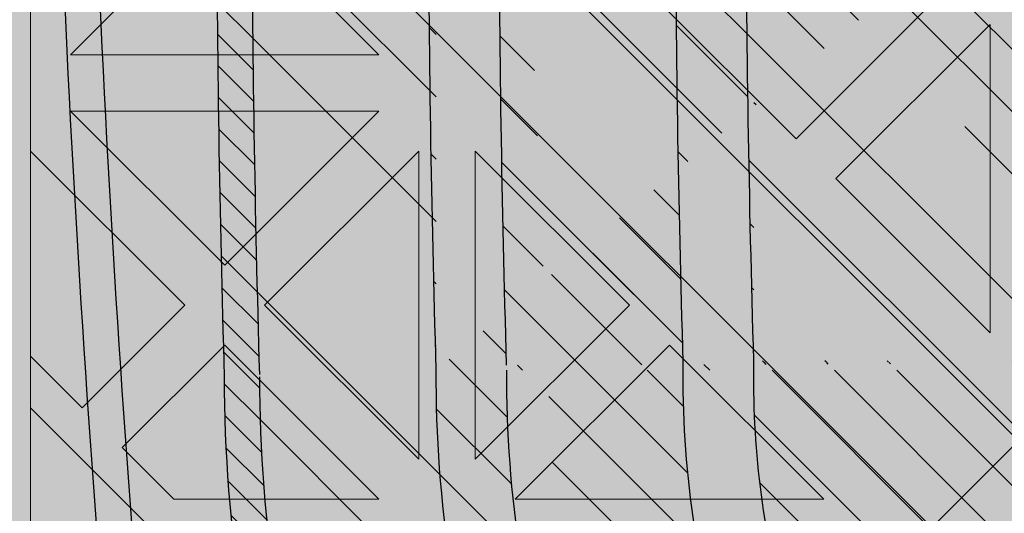
# Model space of a CAD drawing. Units: inches. Extents: x 844 to 2234, y 346 to 1084.
# Tile 28 of 93: x 1252.862 to 1257.311, y 691.183 to 693.415. Entities that reach past the tile are written whole.
import ezdxf

# ---------------------------------------------------------------- set-up
doc = ezdxf.new("R2010")
doc.units = ezdxf.units.IN
doc.header["$MEASUREMENT"] = 0
doc.layers.add('furniture', color=8, linetype='Continuous', lineweight=18)
doc.layers.add('RA-AP-01$0$INT', color=35, linetype='Continuous', lineweight=5)
doc.layers.add('RA-AP-01$0$FURN', color=3, linetype='Continuous')
doc.layers.add('RA-AP-01$0$WOOD', color=64, linetype='Continuous')

# ---------------------------------------------------------------- blocks, each defined once
blk = doc.blocks.new('A$C18D01794')
at = {"layer": 'RA-AP-01$0$INT'}
blk.add_hatch(color=256, dxfattribs=at).paths.add_polyline_path([(4.505206456958071, -6.306712009588038), (5.305206456958072, -6.306712009588038), (5.305206456958072, -7.106712009588038), (5.255206456951893, -7.10671200958804), (5.25520645694868, -6.356712009605972), (4.555206456959269, -6.356712009587461), (4.555206456956052, -7.106712009588038), (4.505206456958073, -7.106712009588038)])
h = blk.add_hatch(color=256, dxfattribs=at)
h.paths.add_polyline_path([(4.585917135068449, -6.356712009588271), (4.555206456959269, -6.35671200958746), (4.555206456959137, -6.387422687716308), (4.874495778835233, -6.706712009592356), (4.90520645695423, -6.676001331474049)])
h.paths.add_polyline_path([(5.255206456948813, -6.387422687716306), (5.255206456948682, -6.356712009605972), (5.224495778822613, -6.356712009605161), (4.905206456953498, -6.676001331474273), (4.935917135072151, -6.706712009592924)])
h.paths.add_polyline_path([(4.935917135072559, -6.706712009592068), (4.905206456953564, -6.737422687710376), (5.255206456951813, -7.087422687708613), (5.255206456951549, -7.026001331471008)])
h.paths.add_polyline_path([(4.555206456956399, -7.026001331471013), (4.555206456956134, -7.087422687708616), (4.905206456953821, -6.737422687710943), (4.874495778835166, -6.70671200959229)])
h = blk.add_hatch(color=256, dxfattribs=at)
h.paths.add_polyline_path([(4.585917135068448, -6.356712009588273), (4.614201406330596, -6.356712009589021), (4.668846067270487, -6.411356670531338), (4.723490728212344, -6.356712009591912), (4.771774999457151, -6.35671200959319), (4.826419660396886, -6.411356670535356), (4.862780050090322, -6.374996280843536), (4.844495778842715, -6.356712009595112), (4.862780050090411, -6.356712009595595), (4.905206456960182, -6.399138416468211), (4.947632863832445, -6.356712009597838), (4.965917135079675, -6.356712009598322), (4.947632863831759, -6.374996280845421), (4.983993253523576, -6.411356670538857), (5.038637914464627, -6.356712009600247), (5.08692218571208, -6.356712009601523), (5.141566846649976, -6.411356670541852), (5.196211507589851, -6.356712009604411), (5.224495778822615, -6.356712009605161), (4.905206456953975, -6.676001331473793)])
h.paths.add_polyline_path([(4.895206456956031, -6.637717060225675), (4.895206456958921, -6.528427738347902), (4.840561796018589, -6.583072399285802)], flags=16)
h.paths.add_polyline_path([(4.915206456955638, -6.637717060226121), (4.969851117895509, -6.583072399288678), (4.915206456957609, -6.528427738348344)], flags=16)
h.paths.add_polyline_path([(4.826419660395175, -6.568930263661755), (4.881064321335613, -6.514285602723745), (4.771774999456703, -6.514285602720857)], flags=16)
h.paths.add_polyline_path([(4.983993253519558, -6.568930263665262), (5.038637914460456, -6.514285602726792), (4.929348592581548, -6.514285602724816)], flags=16)
h.paths.add_polyline_path([(4.881064321336025, -6.494285602723742), (4.826419660397532, -6.439640941782821), (4.771774999457062, -6.494285602720859)], flags=16)
h.paths.add_polyline_path([(4.929348592582019, -6.494285602724817), (5.038637914460982, -6.494285602726792), (4.983993253522945, -6.439640941786327)], flags=16)
h.paths.add_polyline_path([(4.895206456960191, -6.480143467100443), (4.895206456962115, -6.407422687715913), (4.876922185715016, -6.389138416467584), (4.840561796021581, -6.425498806159401)], flags=16)
h.paths.add_polyline_path([(4.915206456958487, -6.480143467100889), (4.969851117899527, -6.425498806162279), (4.933490728206909, -6.389138416468043), (4.9152064569598, -6.40742268771434)], flags=16)
h.paths.add_polyline_path([(4.757632863832376, -6.480143467096812), (4.812277524772842, -6.425498806158772), (4.757632863834348, -6.370854145217844)], flags=16)
h.paths.add_polyline_path([(4.737632863832376, -6.480143467096286), (4.737632863834348, -6.370854145217375), (4.682988202893906, -6.425498806155385)], flags=16)
h.paths.add_polyline_path([(5.05278005008503, -6.480143467103376), (5.052780050087917, -6.370854145224413), (4.998135389146995, -6.425498806162908)], flags=16)
h.paths.add_polyline_path([(5.072780050085024, -6.480143467103744), (5.127424711025931, -6.42549880616527), (5.072780050087916, -6.370854145224832)], flags=16)
h.paths.add_polyline_path([(4.935917135072783, -6.706712009592292), (5.255206456948811, -6.387422687716309), (5.255206456948932, -6.415706958964177), (5.200561796010279, -6.470351619902839), (5.255206456949403, -6.524996280841948), (5.25520645694961, -6.5732805520894), (5.200561796009787, -6.627925213029239), (5.236922185702417, -6.664285602721864), (5.255206456949919, -6.646001331474357), (5.255206456949998, -6.664285602721898), (5.212780050078687, -6.706712009592262), (5.25520645695036, -6.749138416463932), (5.255206456950438, -6.767422687711313), (5.236922185702424, -6.749138416463297), (5.200561796009796, -6.785498806155928), (5.255206456950753, -6.840143467096874), (5.25520645695096, -6.888427738341682), (5.200561796010322, -6.943072399282328), (5.255206456951428, -6.997717060223427), (5.255206456951547, -7.026001331471006)])
h.paths.add_polyline_path([(5.042988202883395, -6.785498806155427), (5.097632863823085, -6.840143467095101), (5.097632863822622, -6.730854145216193)], flags=16)
h.paths.add_polyline_path([(5.028846067259663, -6.771356670531693), (5.083490728198774, -6.716712009592573), (4.974201406321001, -6.716712009593042)], flags=16)
h.paths.add_polyline_path([(5.117632863823087, -6.840143467095186), (5.172277524762331, -6.785498806155926), (5.11763286382262, -6.730854145216225)], flags=16)
h.paths.add_polyline_path([(5.08349072819877, -6.696712009593886), (5.028846067259652, -6.642067348654775), (4.974201406320998, -6.696712009593438)], flags=16)
h.paths.add_polyline_path([(5.131774999446817, -6.854285602718917), (5.186419660386065, -6.799640941779662), (5.241064321325782, -6.854285602719365)], flags=17)
h.paths.add_polyline_path([(5.131774999446228, -6.716712009592374), (5.186419660386065, -6.771356670532194), (5.222780050079488, -6.734996280838764), (5.204495778832781, -6.716712009592063)], flags=16)
h.paths.add_polyline_path([(5.097632863822613, -6.682569873970264), (5.097632863823061, -6.573280552091354), (5.042988202883383, -6.627925213031044)], flags=16)
h.paths.add_polyline_path([(5.131774999446899, -6.874285602718915), (5.241064321325809, -6.874285602719364), (5.186419660386591, -6.928930263658598)], flags=17)
h.paths.add_polyline_path([(5.131774999446226, -6.696712009594078), (5.204495778830767, -6.696712009594374), (5.22278005007868, -6.67842773834687), (5.186419660386049, -6.642067348654249)], flags=16)
h.paths.add_polyline_path([(5.11763286382262, -6.682569873970225), (5.17227752476232, -6.627925213030515), (5.117632863823064, -6.573280552091267)], flags=16)
h.paths.add_polyline_path([(5.186419660386069, -6.613783077405491), (5.241064321325754, -6.559138416465795), (5.131774999446791, -6.559138416466263)], flags=16)
h.paths.add_polyline_path([(5.131774999446872, -6.539138416466263), (5.24106432132578, -6.539138416465794), (5.186419660386554, -6.484493755526573)], flags=16)
h.paths.add_polyline_path([(5.255206456951811, -7.08742268770861), (5.255206456951895, -7.106712009588038), (4.555206456956052, -7.106712009588038), (4.555206456956136, -7.087422687708617), (4.905206456953973, -6.737422687710788)])
h.paths.add_polyline_path([(4.983993253513404, -6.8444937555241), (4.92934859257295, -6.899138416462108), (5.03863791445186, -6.899138416465014)], flags=16)
h.paths.add_polyline_path([(4.969851117889988, -6.83035161990006), (4.915206456952556, -6.775706958960171), (4.915206456949648, -6.884996280837944)], flags=16)
h.paths.add_polyline_path([(4.929348592572535, -6.919138416462105), (4.983993253511019, -6.973783077403037), (5.038637914451496, -6.919138416465012)], flags=16)
h.paths.add_polyline_path([(5.052780050074912, -6.93328055208906), (4.998135389134438, -6.987925213027088), (5.052780050072919, -7.042569873968025)], flags=16)
h.paths.add_polyline_path([(5.07278005007491, -6.933280552089588), (5.072780050072918, -7.042569873968497), (5.127424711013374, -6.987925213030498)], flags=16)
h.paths.add_polyline_path([(4.89520645695295, -6.775706958959721), (4.840561796013067, -6.830351619897157), (4.895206456950961, -6.884996280837494)], flags=16)
h.paths.add_polyline_path([(4.915206456948365, -6.933280552085403), (4.915206456946434, -7.006001331471951), (4.933490728192729, -7.024285602719066), (4.969851117886972, -6.987925213026453)], flags=16)
h.paths.add_polyline_path([(4.881064321327021, -6.899138416461022), (4.82641966038902, -6.84449375552057), (4.771774999448108, -6.899138416459029)], flags=16)
h.paths.add_polyline_path([(4.895206456950073, -6.933280552084951), (4.840561796009022, -6.987925213023558), (4.876922185700835, -7.024285602716997), (4.895206456948749, -7.006001331469487)], flags=16)
h.paths.add_polyline_path([(4.983993253510392, -7.0020673486505), (4.947632863816944, -7.038427738342319), (4.965917135064043, -7.05671200959023), (5.038637914448995, -7.056712009591555)], flags=16)
h.paths.add_polyline_path([(4.881064321326543, -6.91913841646102), (4.771774999447578, -6.919138416459031), (4.826419660385607, -6.973783077399508)], flags=16)
h.paths.add_polyline_path([(4.905206456946447, -7.014285602717636), (4.862780050074785, -7.056712009588352), (4.947632863816685, -7.056712009589775)], flags=16)
h.paths.add_polyline_path([(5.14156684663679, -7.002067348654549), (5.086922185696452, -7.056712009592438), (5.196211507574223, -7.056712009594425)], flags=16)
h.paths.add_polyline_path([(4.8264196603837, -7.002067348646972), (4.771774999442643, -7.056712009585575), (4.8444957788276, -7.056712009587508), (4.862780050075511, -7.038427738340416)], flags=16)
h.paths.add_polyline_path([(4.812277524760289, -6.98792521302292), (4.757632863822258, -6.933280552082447), (4.757632863819352, -7.042569873961408)], flags=16)
h.paths.add_polyline_path([(4.73763286382226, -6.933280552082079), (4.682988202881349, -6.987925213020536), (4.737632863819352, -7.04256987396099)], flags=16)
h.paths.add_polyline_path([(4.723490728195188, -7.056712009584289), (4.668846067257299, -7.002067348643949), (4.614201406317417, -7.056712009581383)], flags=16)
h.paths.add_polyline_path([(4.597632863829262, -6.706712009592262), (4.555206456957951, -6.664285602721896), (4.555206456958029, -6.646001331474357), (4.573490728205535, -6.664285602721864), (4.609851117898167, -6.627925213029238), (4.555206456958338, -6.573280552089402), (4.555206456958546, -6.524996280841952), (4.60985111789767, -6.470351619902839), (4.555206456959015, -6.415706958964177), (4.555206456959138, -6.387422687716309), (4.874495778835167, -6.70671200959229), (4.5552064569564, -7.026001331471015), (4.555206456956523, -6.997717060223433), (4.609851117897629, -6.94307239928233), (4.555206456956988, -6.888427738341681), (4.555206456957198, -6.840143467096881), (4.609851117898153, -6.78549880615593), (4.573490728205528, -6.749138416463297), (4.555206456957507, -6.76742268771132), (4.555206456957585, -6.749138416463933)])
h.paths.add_polyline_path([(4.712780050085332, -6.730854145216195), (4.712780050084863, -6.840143467095105), (4.767424711024555, -6.785498806155427)], flags=16)
h.paths.add_polyline_path([(4.726922185709173, -6.716712009592573), (4.781566846648288, -6.771356670531693), (4.836211507586949, -6.716712009593043)], flags=16)
h.paths.add_polyline_path([(4.692780050085327, -6.730854145216225), (4.638135389145619, -6.785498806155928), (4.692780050084865, -6.840143467095185)], flags=16)
h.paths.add_polyline_path([(4.726922185709182, -6.696712009593886), (4.836211507586949, -6.696712009593436), (4.7815668466483, -6.642067348654773)], flags=16)
h.paths.add_polyline_path([(4.678637914461726, -6.71671200959237), (4.605917135075169, -6.716712009592063), (4.587632863828464, -6.734996280838766), (4.623993253521887, -6.771356670532195)], flags=16)
h.paths.add_polyline_path([(4.712780050085336, -6.68256987397026), (4.767424711024568, -6.627925213031042), (4.71278005008489, -6.573280552091352)], flags=16)
h.paths.add_polyline_path([(4.678637914461726, -6.696712009594076), (4.623993253521899, -6.642067348654247), (4.587632863829271, -6.67842773834687), (4.605917135077185, -6.696712009594376)], flags=16)
h.paths.add_polyline_path([(4.692780050085336, -6.682569873970228), (4.692780050084889, -6.573280552091267), (4.638135389145632, -6.627925213030515)], flags=16)
h.paths.add_polyline_path([(4.623993253521885, -6.799640941779662), (4.678637914461131, -6.854285602718915), (4.56934859258217, -6.854285602719365)], flags=17)
h.paths.add_polyline_path([(4.623993253521901, -6.613783077405509), (4.678637914461158, -6.559138416466263), (4.569348592582195, -6.559138416465795)], flags=16)
h.paths.add_polyline_path([(4.678637914461051, -6.874285602718915), (4.623993253521361, -6.928930263658598), (4.569348592582143, -6.874285602719364)], flags=17)
h.paths.add_polyline_path([(4.678637914461076, -6.539138416466263), (4.623993253521399, -6.484493755526573), (4.569348592582167, -6.539138416465796)], flags=16)
h = blk.add_hatch(color=256, dxfattribs=at)
h.paths.add_polyline_path([(5.028846067259997, -6.642067348655121), (4.974201406321342, -6.696712009593783), (5.083490728199115, -6.69671200959423)])
h.paths.add_polyline_path([(4.974201406321344, -6.716712009593388), (5.028846067260004, -6.771356670532039), (5.083490728199117, -6.716712009592919)])
h.paths.add_polyline_path([(5.042988202883738, -6.785498806155768), (5.097632863823428, -6.840143467095449), (5.097632863822963, -6.73085414521654)])
h.paths.add_polyline_path([(5.117632863822961, -6.730854145216568), (5.117632863823428, -6.840143467095531), (5.172277524762674, -6.785498806156272)])
h.paths.add_polyline_path([(5.131774999446572, -6.716712009592718), (5.186419660386406, -6.77135667053254), (5.222780050079831, -6.734996280839116), (5.204495778833122, -6.716712009592409)])
h.paths.add_polyline_path([(5.236922185702764, -6.749138416463644), (5.200561796010139, -6.785498806156274), (5.255206456949971, -6.840143467096101), (5.255206456950271, -6.76742268771115)])
h.paths.add_polyline_path([(5.186419660386412, -6.799640941780006), (5.131774999447164, -6.854285602719262), (5.241064321326123, -6.854285602719711)])
h.paths.add_polyline_path([(5.131774999447238, -6.874285602719261), (5.186419660386934, -6.928930263658944), (5.241064321326153, -6.874285602719709)])
h.paths.add_polyline_path([(5.200561796010663, -6.943072399282675), (5.255206456949324, -6.997717060221329), (5.255206456949777, -6.888427738343558)])
h.paths.add_polyline_path([(5.21278005007903, -6.706712009592607), (5.255206456950223, -6.749138416463798), (5.255206456950696, -6.664285602721891)])
h.paths.add_polyline_path([(5.13177499944657, -6.696712009594424), (5.204495778831106, -6.696712009594723), (5.222780050079024, -6.678427738347219), (5.186419660386397, -6.642067348654592)])
h.paths.add_polyline_path([(5.117632863823405, -6.573280552091611), (5.117632863822955, -6.682569873970578), (5.172277524762665, -6.627925213030859)])
h.paths.add_polyline_path([(5.042988202883727, -6.627925213031387), (5.097632863822957, -6.682569873970603), (5.097632863823407, -6.573280552091697)])
h.paths.add_polyline_path([(5.131774999447135, -6.559138416466609), (5.186419660386394, -6.613783077405857), (5.241064321326097, -6.559138416466144)])
h.paths.add_polyline_path([(5.200561796010128, -6.627925213029584), (5.236922185702758, -6.664285602722211), (5.255206456950264, -6.646001331474705), (5.255206456949948, -6.573280552089752)])
h.paths.add_polyline_path([(5.186419660386895, -6.484493755526919), (5.131774999447213, -6.539138416466609), (5.241064321326127, -6.539138416466142)])
h.paths.add_polyline_path([(5.200561796010624, -6.470351619903183), (5.255206456949745, -6.524996280842298), (5.255206456949276, -6.415706958964523)])
h = blk.add_hatch(color=256, dxfattribs=at)
h.paths.add_polyline_path([(4.905206456953579, -6.70671200959253), (4.905206456953751, -6.676001331474523), (4.874495778835229, -6.706712009592358)])
h.paths.add_polyline_path([(4.935917135071924, -6.706712009592703), (4.905206456953583, -6.706712009592529), (4.90520645695341, -6.737422687710532)])
h = blk.add_hatch(color=256, dxfattribs=at)
h.paths.add_polyline_path([(4.895206456952951, -6.77570695895972), (4.840561796013068, -6.830351619897156), (4.895206456950958, -6.884996280837495)])
h.paths.add_polyline_path([(4.915206456949649, -6.884996280837942), (4.969851117889987, -6.830351619900054), (4.915206456952556, -6.775706958960171)])
h.paths.add_polyline_path([(5.038637914451862, -6.899138416465013), (4.983993253513403, -6.8444937555241), (4.929348592572953, -6.899138416462106)])
h.paths.add_polyline_path([(4.929348592572535, -6.919138416462105), (4.983993253511018, -6.973783077403037), (5.038637914451497, -6.919138416465012)])
h.paths.add_polyline_path([(4.915206456948366, -6.933280552085397), (4.915206456946433, -7.006001331471951), (4.93349072819273, -7.024285602719068), (4.969851117886972, -6.987925213026454)])
h.paths.add_polyline_path([(5.038637914448995, -7.056712009591553), (4.983993253510389, -7.002067348650502), (4.947632863816946, -7.038427738342318), (4.965917135064043, -7.05671200959023)])
h.paths.add_polyline_path([(5.05278005007292, -7.042569873968023), (5.05278005007491, -6.933280552089059), (4.998135389134438, -6.987925213027088)])
h.paths.add_polyline_path([(5.07278005007292, -7.042569873968496), (5.127424711013374, -6.987925213030498), (5.072780050074909, -6.933280552089588)])
h.paths.add_polyline_path([(5.141566846636789, -7.002067348654547), (5.086922185696449, -7.056712009592438), (5.196211507574223, -7.056712009594425)])
h.paths.add_polyline_path([(4.947632863816688, -7.056712009589774), (4.905206456946449, -7.014285602717634), (4.862780050074784, -7.056712009588353)])
h.paths.add_polyline_path([(4.840561796009025, -6.987925213023556), (4.876922185700834, -7.024285602716997), (4.895206456948747, -7.006001331469488), (4.895206456950075, -6.933280552084953)])
h.paths.add_polyline_path([(4.88106432132654, -6.919138416461021), (4.771774999447577, -6.919138416459031), (4.826419660385606, -6.973783077399508)])
h.paths.add_polyline_path([(4.881064321327019, -6.899138416461022), (4.826419660389019, -6.844493755520571), (4.771774999448108, -6.89913841645903)])
h.paths.add_polyline_path([(4.757632863819352, -7.042569873961409), (4.812277524760284, -6.987925213022922), (4.757632863822259, -6.933280552082447)])
h.paths.add_polyline_path([(4.8264196603837, -7.002067348646974), (4.771774999442646, -7.056712009585575), (4.844495778827599, -7.05671200958751), (4.862780050075512, -7.038427738340417)])
h.paths.add_polyline_path([(4.737632863819352, -7.042569873960988), (4.737632863822258, -6.933280552082078), (4.682988202881349, -6.987925213020538)])
h.paths.add_polyline_path([(4.668846067257299, -7.002067348643952), (4.61420140631742, -7.056712009581384), (4.723490728195189, -7.056712009584292)])
for p, q in [((5.255206456951895, -7.106712009588038), (5.255206456948681, -6.356712009605972)), ((5.25520645694988, -6.74913841646345), (5.255206456950353, -6.664285602721543)), ((4.935917135071927, -6.706712009592701), (4.905206456953407, -6.737422687710532)), ((4.935917135072783, -6.706712009592292), (5.255206456951548, -7.026001331471007)), ((5.212780050078687, -6.706712009592262), (5.25520645694988, -6.74913841646345)), ((5.083490728198772, -6.716712009592574), (4.974201406321001, -6.716712009593042)), ((4.974201406321001, -6.716712009593042), (5.028846067259663, -6.771356670531693)), ((5.08349072819877, -6.716712009592578), (5.028846067259663, -6.771356670531693)), ((5.131774999446229, -6.716712009592372), (5.186419660386063, -6.771356670532195)), ((5.204495778831181, -6.716712009592063), (5.131774999446229, -6.716712009592372)), ((5.204495778832774, -6.716712009592056), (5.222780050080282, -6.73499628083956)), ((5.09763286382262, -6.730854145216195), (5.042988202883395, -6.785498806155425)), ((5.097632863823085, -6.840143467095105), (5.09763286382262, -6.730854145216195)), ((5.11763286382262, -6.730854145216223), (5.172277524762331, -6.785498806155928)), ((5.117632863823085, -6.840143467095186), (5.11763286382262, -6.730854145216223)), ((5.186419660386062, -6.771356670532195), (5.222780050078687, -6.734996280839565)), ((4.905206456953975, -6.737422687710788), (5.255206456951811, -7.087422687708611)), ((5.200561796009796, -6.78549880615593), (5.236922185702423, -6.749138416463297)), ((5.255206456949928, -6.767422687710803), (5.236922185702423, -6.749138416463296)), ((5.236922185702423, -6.749138416463297), (5.25520645694988, -6.767422687710757)), ((5.255206456949927, -6.767422687710803), (5.255206456949628, -6.840143467095755)), ((4.915206456952556, -6.775706958960171), (4.969851117889986, -6.830351619900053)), ((4.915206456949648, -6.884996280837942), (4.915206456952556, -6.775706958960171)), ((5.042988202883397, -6.785498806155427), (5.097632863823085, -6.840143467095105)), ((5.117632863823085, -6.840143467095186), (5.172277524762331, -6.785498806155928)), ((5.255206456949628, -6.840143467095755), (5.200561796009796, -6.785498806155928)), ((5.131774999446817, -6.854285602718915), (5.186419660386065, -6.799640941779662)), ((5.24106432132578, -6.854285602719365), (5.186419660386065, -6.799640941779662)), ((4.915206456949651, -6.88499628083794), (4.969851117889986, -6.830351619900053)), ((4.929348592572952, -6.899138416462106), (4.983993253513403, -6.844493755524101)), ((4.983993253513404, -6.844493755524103), (5.038637914451862, -6.899138416465012)), ((5.131774999446817, -6.854285602718915), (5.24106432132578, -6.854285602719365)), ((5.131774999446899, -6.874285602718915), (5.241064321325809, -6.874285602719364)), ((5.186419660386587, -6.928930263658596), (5.131774999446899, -6.874285602718915)), ((5.241064321325809, -6.874285602719364), (5.186419660386589, -6.928930263658598))]:
    blk.add_line(p, q, dxfattribs=at)
blk = doc.blocks.new('A$C32926AE1')
at = {"layer": 'RA-AP-01$0$FURN'}
h = blk.add_hatch(dxfattribs=at)
h.set_pattern_fill('ANSI31', color=256, scale=0.1, style=0)
h.set_pattern_definition([(45, (0, 0), (-0.0088388347648318, 0.0088388347648318), [])])
edge = h.paths.add_edge_path(flags=16)
edge.add_arc((4.904771284329206, 4.246793130718756), 0.2603971832811541, 75.22398030683196, 104.7760196931204)
edge.add_arc((4.904771284329206, 4.246793130718756), 0.2603971832811541, 75.223980306832, 104.77601969312039, ccw=False)
edge = h.paths.add_edge_path(flags=16)
edge.add_arc((4.904771284329206, 4.067062675376612), 0.2603971832811541, 255.2239803068796, 284.776019693168)
edge.add_arc((4.904771284329206, 4.067062675376612), 0.2603971832811541, 255.22398030687958, 284.77601969316805, ccw=False)
edge = h.paths.add_edge_path(flags=0)
edge.add_arc((4.904771284329206, 4.067062675376612), 0.2603971832811541, 255.2239803068796, 284.776019693168)
edge.add_arc((4.904771284329206, 4.067062675376612), 0.2603971832811541, 255.22398030687958, 284.77601969316805, ccw=False)
edge = h.paths.add_edge_path(flags=0)
edge.add_arc((4.904771284329206, 4.067062675376612), 0.2603971832811541, 255.2239803068796, 284.776019693168)
edge.add_arc((4.904771284329206, 4.067062675376612), 0.2603971832811541, 255.22398030687958, 284.77601969316805, ccw=False)
edge = h.paths.add_edge_path()
edge.add_arc((4.604388392048174, 4.588829985554312), 0.1599999999999918, 342.3781640246255, 354.4317409793762)
edge.add_arc((5.090145208887507, 4.43216705527679), 0.3503971832811637, 162.0091218307731, 180.3186872093483)
edge.add_arc((5.205154176610243, 4.588829985554953), 0.1599999999999917, 185.5682590208461, 197.6218359767349)
edge.add_arc((4.904771284329229, 4.246793130718735), 0.3503971832811761, 72.00912183053516, 107.9908781690354)
edge.add_arc((9.535952835716557, 4.28682295566602), 4.798342501046485, 178.2875002453811, 181.5576802719453)
edge.add_arc((4.719397359771122, 4.43216705527679), 0.3503971832811637, 359.6813127906516, 377.9908781692269)
edge.add_arc((9.535967292294904, 4.286822350292874), 4.778371420254705, 178.2965938931842, 181.5667745797229)
edge.add_arc((4.719397359771122, 4.43216705527679), 0.3303971832811637, 359.6813127906516, 377.9908781692269)
edge.add_arc((0.2735752763637294, 4.286822350292874), 4.7783714202547, 358.4332254202771, 361.7034061068158)
edge.add_arc((5.061434214606998, 4.732549947558029), 0.1600000000000254, 252.3781640250584, 264.4317409792362)
edge.add_arc((4.748108354051257, 4.732549947558012), 0.1600000000000541, 275.5682590208426, 287.6218359759532)
edge.add_arc((4.604388392048115, 4.588829985554317), 0.1800000000000505, 342.3567572500182, 349.3735009646207)
edge.add_arc((5.205154176610254, 4.588829985554976), 0.1800000000000069, 190.6264990356027, 197.6432427513933)
edge.add_arc((5.061434214607106, 4.732549947558013), 0.1800000000000424, 252.3567572496606, 259.3735009644582)
edge.add_arc((4.904771284329208, 4.246793130718737), 0.3303971832811676, 71.99844483668534, 108.0015551637021)
edge.add_arc((4.748108354051414, 4.732549947558045), 0.1800000000000547, 280.6264990355479, 287.6432427495938)
edge.add_arc((5.090145208887514, 4.432167055276789), 0.2803971832811691, 162.8706300666893, 180.816523289902)
edge.add_arc((4.719397359771136, 4.432167055276689), 0.2803971832811534, 359.183476710103, 377.1293699333214)
edge.add_arc((4.904771284329222, 4.246793130718737), 0.2803971832811769, 72.87063006672916, 107.1293699332334)
edge.add_arc((5.090145208887522, 4.432167055276788), 0.2603971832811776, 165.2239803068007, 180.9953123810312)
edge.add_arc((4.719397359771141, 4.432167055276699), 0.2603971832811458, 359.0046876189768, 374.7760196932087)
edge.add_arc((5.090145208887507, 4.43216705527679), 0.3303971832811637, 162.0091218307731, 180.3186872093483)
edge.add_arc((9.53595427642584, 4.285015535491528), 4.728345371032053, 178.265043920078, 181.5679956281801)
edge.add_arc((0.2735882922327999, 4.285015535491582), 4.728345371032045, 358.4320043718193, 361.7349560799204)
edge.add_arc((9.535953591267507, 4.284458026472751), 4.708343996644348, 178.2573054306777, 181.5704995759608)
edge.add_arc((0.273588977391114, 4.284458026472785), 4.708343996644358, 358.4295004240388, 361.7426945693213)
edge.add_arc((0.2735889773911131, 4.029397779622582), 4.708343996644359, 358.2573054306787, 361.5704995759613)
edge.add_arc((9.535953591267518, 4.029397779622618), 4.708343996644359, 178.4295004240391, 181.7426945693223)
edge.add_arc((0.2735882922327901, 4.028840270603786), 4.728345371032054, 358.2650439200796, 361.5679956281808)
edge.add_arc((9.53595427642584, 4.028840270603841), 4.728345371032054, 178.4320043718199, 181.7349560799219)
edge.add_arc((0.2735752763637302, 4.027033455802493), 4.778371420254699, 358.2965938931842, 361.5667745797229)
edge.add_arc((4.719397359771122, 3.881688750818578), 0.3303971832811637, 342.0091218307731, 360.3186872093484)
edge.add_arc((5.090145208887507, 3.881688750818578), 0.3303971832811637, 179.6813127906516, 197.9908781692269)
edge.add_arc((9.535967292294904, 4.027033455802493), 4.778371420254705, 178.433225420277, 181.7034061068158)
edge.add_arc((4.719397359771122, 3.881688750818578), 0.3503971832811637, 342.0091218307731, 360.3186872093484)
edge.add_arc((9.53595283571655, 4.027032850429349), 4.79834250104648, 178.4423197280546, 181.7124997546188)
edge.add_arc((4.719397359771141, 3.881688750818669), 0.2603971832811458, 345.2239803067913, 360.9953123810232)
edge.add_arc((5.090145208887522, 3.88168875081858), 0.2603971832811776, 179.0046876189687, 194.7760196931993)
edge.add_arc((4.904771284329222, 4.067062675376631), 0.2803971832811769, 252.8706300667665, 287.1293699332708)
edge.add_arc((4.719397359771136, 3.881688750818678), 0.2803971832811534, 342.8706300666787, 360.8165232898969)
edge.add_arc((5.090145208887514, 3.881688750818579), 0.2803971832811691, 179.183476710098, 197.1293699333106)
edge.add_arc((4.748108354051414, 3.581305858537323), 0.1800000000000547, 72.3567572504062, 79.37350096445199)
edge.add_arc((4.904771284329208, 4.067062675376631), 0.3303971832811676, 251.9984448362979, 288.0015551633146)
edge.add_arc((5.061434214607106, 3.581305858537355), 0.1800000000000424, 100.6264990355418, 107.6432427503394)
edge.add_arc((5.205154176610254, 3.725025820540392), 0.1800000000000069, 162.3567572486066, 169.3735009643972)
edge.add_arc((4.604388392048115, 3.725025820541051), 0.1800000000000505, 10.62649903537925, 17.64324274998182)
edge.add_arc((4.748108354051257, 3.581305858537356), 0.1600000000000541, 72.37816402404681, 84.43174097915735)
edge.add_arc((4.904771284329229, 4.067062675376632), 0.3503971832811761, 252.0091218309645, 287.9908781694648)
edge.add_arc((5.061434214606998, 3.581305858537339), 0.1600000000000254, 95.56825902076373, 107.6218359749416)
edge.add_arc((5.205154176610243, 3.725025820540414), 0.1599999999999917, 162.3781640232651, 174.4317409791539)
edge.add_arc((5.090145208887507, 3.881688750818578), 0.3503971832811637, 179.6813127906516, 197.9908781692269)
edge.add_arc((4.604388392048174, 3.725025820541056), 0.1599999999999918, 5.568259020623824, 17.62183597537444)
edge.add_arc((0.2735897329420762, 4.28682295566602), 4.798342501046482, 358.4423197280547, 361.7124997546188)
edge.add_arc((0.2735897329420691, 4.027032850429348), 4.798342501046489, 358.2875002453812, 361.5576802719453)
at = {"layer": 'RA-AP-01$0$WOOD'}
h = blk.add_hatch(color=256, dxfattribs=at)
h.dxf.hatch_style = 1
h.paths.add_polyline_path([(5.157430609644524, 4.573483066760929, -0.1009492694046607), (5.155401577623758, 4.593365984175333, -0.1842662638101597), (5.172249623284174, 4.638795604568598, 0.2056608120311276), (5.179560981299304, 4.661316324430096, 0.3614336704623542), (5.134352340494423, 4.706524965234944, 0.2056608120311297), (5.111831620632933, 4.699213607219793, -0.1842662638101113), (5.066402000239693, 4.682365561559342, -0.1055311479399994), (5.045656153913092, 4.68467289944697, 0.1567636581983829), (4.763886414745334, 4.684672899446966, -0.1055311479399895), (4.743140568418733, 4.68236556155934, -0.1842662638100833), (4.6977109480255, 4.69921360721979, 0.2056608120302612), (4.675190228164109, 4.706524965234949, 0.3614336704708441), (4.629981587358889, 4.66131632442871, 0.2056608120245944), (4.637292945374126, 4.638795604567974, -0.1842662638101024), (4.654140991034615, 4.59336598417475, -0.1009492694055169), (4.652111959013835, 4.573483066760181, 0.021410119221476), (4.629748025606143, 4.156712009541676, 0.0214101192214795), (4.652111959013809, 3.739940952323101, -0.1009492694059586), (4.654140991034615, 3.720058034908448, -0.1842662638100975), (4.637292945374126, 3.674628414515226, 0.2056608120245705), (4.629981587358889, 3.652107694654492, 0.3614336704708879), (4.675190228164113, 3.606899053848249, 0.2056608120302384), (4.697710948025501, 3.614210411863408, -0.1842662638100995), (4.743140568418738, 3.63105845752386, -0.1055311479402541), (4.763886414745388, 3.628751119636215, 0.1567636581983776), (5.045656153913137, 3.628751119636244, -0.1055311479397538), (5.066402000239692, 3.631058457523857, -0.1842662638101067), (5.111831620632931, 3.614210411863407, 0.2056608120310924), (5.134352340494417, 3.606899053848256, 0.3614336704624001), (5.179560981299307, 3.652107694653103, 0.2056608120311314), (5.172249623284175, 3.6746284145146, -0.1842662638101402), (5.155401577623758, 3.72005803490786, -0.1009492694051366), (5.15743060964455, 3.739940952322354, 0.0214101192215073), (5.179794543052287, 4.156712009541468, 0.0214101192215252)])
h.paths.add_polyline_path([(4.639748609479751, 4.156712009541513, 0.0213537860821624), (4.661970494867118, 3.741887061152232, -0.094075836301374), (4.664143710413708, 3.7196126951003, -0.1824818158568985), (4.644813765429836, 3.668037719127816, 0.2056608120245319), (4.639939526753007, 3.653023905887301, 0.3614336704710246), (4.676106439397173, 3.616856993242342, 0.2056608120302234), (4.691120252638095, 3.621731231919122, -0.1824818158602558), (4.742695228611606, 3.641061176902986, -0.1029891339458722), (4.766991894714349, 3.638256818950944, 0.156709409989566), (5.042550673941472, 3.638256818950105, -0.102989133958497), (5.066847340047078, 3.641061176902949, -0.1824818158594995), (5.118422316020358, 3.621731231919103, 0.2056608120311416), (5.133436129261316, 3.616856993242346, 0.3614336704621468), (5.169603041905217, 3.653023905886178, 0.2056608120310986), (5.164728803228477, 3.668037719127177, -0.1824818158565612), (5.145398858244737, 3.719612695099578, -0.0940758363009313), (5.147572073791232, 3.741887061151398, 0.0213537860822023), (5.169793959178681, 4.156712009541451, 0.0213537860822226), (5.147572073791203, 4.571536957931898, -0.0940758363005034), (5.145398858244737, 4.59381132398362, -0.1824818158565587), (5.164728803228476, 4.645386299956021, 0.2056608120311045), (5.169603041905216, 4.66040011319702, 0.3614336704621845), (5.133436129261313, 4.696567025840856, 0.2056608120310773), (5.118422316020359, 4.691692787164098, -0.182481815859508), (5.066847340047078, 4.67236284218025, -0.1029891339584606), (5.04255067394148, 4.675167200133092, 0.156709409989566), (4.766991894714357, 4.675167200132257, -0.1029891339458842), (4.742695228611611, 4.672362842180213, -0.1824818158602725), (4.691120252638095, 4.691692787164077, 0.2056608120302152), (4.676106439397174, 4.696567025840858, 0.3614336704710363), (4.639939526753005, 4.660400113195899, 0.2056608120245495), (4.644813765429837, 4.645386299955384, -0.1824818158568934), (4.664143710413708, 4.593811323982902, -0.0940758363009187), (4.661970494867149, 4.571536957931074, 0.021353786082177)], flags=16)
h.paths.add_polyline_path([(5.129794543052235, 4.432167055276933, -0.0141661062790638), (5.130152669293814, 4.156927903047693, -0.0141661062790647), (5.129794543052234, 3.881688750818433, -0.0785247771143638), (5.10979738006795, 3.755143611847103, 0.0945969212073497), (5.105408519571111, 3.717898134952927, 0.1043170707844957), (5.116074640131521, 3.670385395016088, 0.1043170707864965), (5.068561900193738, 3.681051515576561, 0.09459692119553), (5.031316423304057, 3.676662655080835, -0.1580239521427272), (4.778226145355827, 3.676662655080367, 0.0945969211986668), (4.740980668464973, 3.681051515576592, 0.1043170707882822), (4.693467928526415, 3.670385395015844, 0.1043170707867916), (4.704134049087309, 3.717898134953662, 0.0945969211972894), (4.69974518859162, 3.755143611844042, -0.0785247771163196), (4.679748025606343, 3.881688750818406, -0.0141661062790663), (4.679389899364763, 4.156927903047693, -0.0141661062790672), (4.679748025606343, 4.432167055276998, -0.0785247771163064), (4.699745188591625, 4.55871219425134, 0.094596921197333), (4.704134049087308, 4.595957671141738, 0.1043170707867205), (4.693467928526416, 4.643470411079523, 0.1043170707882628), (4.740980668464965, 4.632804290518776, 0.0945969211988114), (4.778226145355874, 4.637193151015016, -0.158023952142669), (5.031316423304015, 4.637193151014546, 0.0945969211956361), (5.068561900193736, 4.632804290518806, 0.1043170707864979), (5.11607464013152, 4.643470411079278, 0.1043170707844617), (5.105408519571112, 4.595957671142455, 0.0945969212074597), (5.109797380067959, 4.558712194248236, -0.0785247771143467)], flags=0)
h.paths.add_polyline_path([(5.119794532311105, 4.432259799204851, -0.0142000800617244), (5.120156169157484, 4.156927903047701, -0.0142000800617277), (5.119794532311105, 3.881596006890482, -0.0784894509520253), (5.100273383573699, 3.758192358677797, 0.0940138827242913), (5.095413455884425, 3.717477693979438, 0.0606271852308753), (5.099615656341024, 3.686844378806616, 0.0606271852322524), (5.068982341167493, 3.691046579263239, 0.0940138827010453), (5.028267676478798, 3.686186651576848, -0.1580706864508061), (4.781274892180912, 3.686186651576435, 0.0940138827026903), (4.740560227491556, 3.691046579263279, 0.0606271852339895), (4.709926912317155, 3.686844378806508, 0.0606271852329405), (4.714129112773991, 3.717477693980356, 0.094013882701304), (4.709269185087677, 3.758192358669163, -0.0784894509577193), (4.689748036347473, 3.881596006890469, -0.014200080061729), (4.689386399501094, 4.156927903047709, -0.0142000800617217), (4.689748036347473, 4.432259799204808, -0.078489450957724), (4.709269185087651, 4.555663447426125, 0.0940138827014585), (4.714129112773992, 4.596378112114996, 0.0606271852329731), (4.709926912317154, 4.62701142728886, 0.0606271852340196), (4.74056022749157, 4.622809226832087, 0.0940138827024997), (4.781274892180847, 4.627669154518912, -0.1580706864508359), (5.028267676478777, 4.627669154518526, 0.0940138827010946), (5.068982341167492, 4.622809226832129, 0.060627185232254), (5.099615656341024, 4.627011427288751, 0.0606271852308727), (5.095413455884425, 4.59637811211593, 0.0940138827241088), (5.100273383573675, 4.555663447417647, -0.0784894509520978)], flags=0)
h.paths.add_polyline_path([(5.06978912287499, 4.430218106756144, -0.014241683694547), (5.070173729147532, 4.156927903047672, -0.0142416836945458), (5.06978912287499, 3.883637699339223, -0.0800609523125196), (5.052662118612511, 3.773463122773442, 0.0526421978001116), (5.04590916754064, 3.740550867606997, 0.0526421977992423), (5.012996912374707, 3.73379791653534, -0.1583028414718258), (4.796545656286308, 3.73379791653451, 0.0526421978034211), (4.763633401117837, 3.740550867607021, 0.0526421978018622), (4.756880450045755, 3.773463122774558, -0.0800609523117106), (4.739753445783639, 3.883637699339268, -0.0142416836945435), (4.739368839511098, 4.156927903047671, -0.0142416836945477), (4.739753445783639, 4.430218106756155, -0.0800609523116345), (4.75688045004574, 4.540392683320762, 0.052642197801941), (4.763633401117837, 4.573304938488346, 0.0526421978035071), (4.796545656286361, 4.580057889560873, -0.1583028414717561), (5.012996912374669, 4.580057889560039, 0.0526421977993048), (5.04590916754064, 4.57330493848837, 0.0526421978002057), (5.052662118612529, 4.540392683321868, -0.080060952312477)], flags=0)
h.paths.add_polyline_path([(5.049789715110557, 4.43038092723357, -0.0143097550741839), (5.05018085590259, 4.156927903047715, -0.0143097550741854), (5.049789715110558, 3.883474878861827, -0.0800685599149176), (5.03362098255317, 3.779581877367999, 0.0306258898956367), (5.028241146483733, 3.758218888663947, 0.0306258898977031), (5.006878157778253, 3.75283905259408, -0.1583983521624096), (4.802664410878162, 3.752839052594731, 0.0306258898946014), (4.781301422174808, 3.758218888663924, 0.0306258898967912), (4.775921586105202, 3.779581877368794, -0.080068559914251), (4.759752853548071, 3.883474878861786, -0.0143097550741854), (4.759361712756037, 4.156927903047671, -0.0143097550741854), (4.759752853548071, 4.430380927233557, -0.0800685599142479), (4.775921586105193, 4.534273928726546, 0.0306258898968306), (4.781301422174808, 4.555636917431444, 0.0306258898945754), (4.802664410878143, 4.561016753500631, -0.1583983521624168), (5.006878157778244, 4.561016753501291, 0.0306258898977177), (5.028241146483733, 4.555636917431421, 0.0306258898958182), (5.03362098255321, 4.534273928727244, -0.080068559914796)], flags=0)
h.paths.add_polyline_path([(4.999766070382627, 4.428171244713864, -0.0143443147609634), (5.000198441819402, 4.156927903047689, -0.0143443147609612), (4.999766070382627, 3.885684561381556, -0.0784641635803329), (4.987356730658798, 3.799103304488872, -0.1506053783831347), (4.822185837999821, 3.79910330448882, -0.0784641635803318), (4.809776498276007, 3.885684561381509, -0.014344314760963), (4.809344126839227, 4.156927903047677, -0.0143443147609645), (4.809776498276007, 4.428171244713873, -0.0784641635803192), (4.822185837999822, 4.514752501606549, -0.1506053783831338), (4.987356730658798, 4.514752501606494, -0.078464163580285)], flags=0)
h.paths.add_polyline_path([(4.979755254238824, 4.42764379880488, -0.0143772539198268), (4.980205517789977, 4.156927903047693, -0.0143772539198275), (4.979755254238824, 3.886212007290489, -0.0689242507424422), (4.971183264704897, 3.815276770442801, -0.1296645318904179), (4.838359303953726, 3.815276770442746, -0.0689242507424186), (4.829787314419809, 3.886212007290419, -0.0143772539198292), (4.829337050868653, 4.156927903047653, -0.0143772539198325), (4.829787314419809, 4.427643798804946, -0.0689242507424211), (4.838359303953725, 4.498579035652621, -0.1296645318904187), (4.971183264704897, 4.498579035652565, -0.0689242507424401)], flags=0)
h = blk.add_hatch(color=256, dxfattribs=at)
h.dxf.hatch_style = 1
h.paths.add_polyline_path([(5.145398858244737, 4.59381132398362, -0.1824818158565616), (5.164728803228476, 4.645386299956021, 0.2056608120311045), (5.169603041905216, 4.66040011319702, 0.3614336704621845), (5.133436129261313, 4.696567025840856, 0.2056608120310773), (5.118422316020359, 4.691692787164098, -0.182481815859508), (5.066847340047078, 4.67236284218025, -0.1029891339584606), (5.04255067394148, 4.675167200133092, 0.156709409989566), (4.766991894714357, 4.675167200132257, -0.1029891339458842), (4.742695228611611, 4.672362842180213, -0.1824818158602725), (4.691120252638095, 4.691692787164077, 0.2056608120302152), (4.676106439397174, 4.696567025840858, 0.3614336704710363), (4.639939526753005, 4.660400113195899, 0.2056608120245495), (4.644813765429837, 4.645386299955384, -0.1824818158568934), (4.664143710413708, 4.593811323982902, -0.0940758363009187), (4.661970494867149, 4.571536957931074, 0.0213537860821772), (4.639748609479751, 4.156712009541507, 0.0213537860821625), (4.661970494867119, 3.741887061152226, -0.0940758363013071), (4.664143710413708, 3.719612695100309, -0.1824818158569294), (4.644813765429836, 3.668037719127816, 0.2056608120245319), (4.639939526753007, 3.653023905887301, 0.3614336704710246), (4.676106439397173, 3.616856993242342, 0.2056608120302234), (4.691120252638095, 3.621731231919122, -0.1824818158602558), (4.742695228611606, 3.641061176902986, -0.1029891339458722), (4.766991894714349, 3.638256818950944, 0.156709409989566), (5.042550673941472, 3.638256818950105, -0.102989133958497), (5.066847340047078, 3.641061176902949, -0.1824818158594995), (5.118422316020358, 3.621731231919103, 0.2056608120311416), (5.133436129261316, 3.616856993242346, 0.3614336704621468), (5.169603041905217, 3.653023905886178, 0.2056608120310986), (5.164728803228477, 3.668037719127177, -0.1824818158565612), (5.145398858244737, 3.719612695099578, -0.0940758363009313), (5.147572073791232, 3.741887061151398, 0.0213537860822023), (5.169793959178681, 4.156712009541451, 0.0213537860822226), (5.147572073791203, 4.571536957931898, -0.0940758363004996)])
h.paths.add_polyline_path([(5.109797380067958, 4.55871219424824, -0.0785247771143472), (5.129794543052234, 4.432167055276936, -0.0141661062790644), (5.130152669293814, 4.156927903047685, -0.014166106279066), (5.129794543052234, 3.881688750818401, -0.0785247771143517), (5.109797380067946, 3.755143611847092, 0.0945969212073132), (5.105408519571111, 3.717898134952929, 0.1043170707844995), (5.116074640131521, 3.670385395016088, 0.1043170707864965), (5.068561900193738, 3.681051515576561, 0.09459692119553), (5.031316423304057, 3.676662655080835, -0.1580239521427272), (4.778226145355827, 3.676662655080367, 0.0945969211986668), (4.740980668464973, 3.681051515576592, 0.1043170707882822), (4.693467928526415, 3.670385395015844, 0.1043170707867916), (4.704134049087309, 3.717898134953662, 0.0945969211972894), (4.69974518859162, 3.755143611844042, -0.0785247771163196), (4.679748025606343, 3.881688750818406, -0.0141661062790663), (4.679389899364763, 4.156927903047693, -0.0141661062790672), (4.679748025606343, 4.432167055276998, -0.0785247771163064), (4.699745188591625, 4.55871219425134, 0.094596921197333), (4.704134049087308, 4.595957671141738, 0.1043170707867205), (4.693467928526416, 4.643470411079523, 0.1043170707882628), (4.740980668464965, 4.632804290518776, 0.0945969211988114), (4.778226145355874, 4.637193151015016, -0.158023952142669), (5.031316423304015, 4.637193151014546, 0.0945969211956361), (5.068561900193736, 4.632804290518806, 0.1043170707864979), (5.11607464013152, 4.643470411079278, 0.1043170707844617), (5.105408519571112, 4.595957671142455, 0.0945969212074504)], flags=16)
h.paths.add_polyline_path([(5.100273383573655, 4.55566344741771, -0.0784894509521388), (5.119794532311105, 4.432259799204852, -0.0142000800617252), (5.120156169157484, 4.156927903047686, -0.014200080061726), (5.119794532311105, 3.881596006890502, -0.0784894509520446), (5.100273383573696, 3.758192358677786, 0.0940138827242721), (5.095413455884425, 3.717477693979436, 0.0606271852308692), (5.099615656341024, 3.686844378806616, 0.0606271852322522), (5.068982341167493, 3.691046579263239, 0.0940138827010453), (5.028267676478798, 3.686186651576848, -0.1580706864508061), (4.781274892180912, 3.686186651576435, 0.0940138827026903), (4.740560227491556, 3.691046579263279, 0.0606271852339895), (4.709926912317155, 3.686844378806508, 0.0606271852329405), (4.714129112773991, 3.717477693980356, 0.094013882701304), (4.709269185087677, 3.758192358669163, -0.0784894509577193), (4.689748036347473, 3.881596006890469, -0.014200080061729), (4.689386399501094, 4.156927903047709, -0.0142000800617217), (4.689748036347473, 4.432259799204808, -0.078489450957724), (4.709269185087651, 4.555663447426125, 0.0940138827014585), (4.714129112773992, 4.596378112114996, 0.0606271852329731), (4.709926912317154, 4.62701142728886, 0.0606271852340196), (4.74056022749157, 4.622809226832087, 0.0940138827024997), (4.781274892180847, 4.627669154518912, -0.1580706864508359), (5.028267676478777, 4.627669154518526, 0.0940138827010946), (5.068982341167492, 4.622809226832129, 0.060627185232254), (5.099615656341024, 4.627011427288751, 0.0606271852308727), (5.095413455884425, 4.59637811211593, 0.094013882723957)], flags=0)
h.paths.add_polyline_path([(5.04590916754064, 4.57330493848837, 0.0526421978002057), (5.052662118612529, 4.540392683321868, -0.0800609523124783), (5.06978912287499, 4.430218106756142, -0.0142416836945469), (5.070173729147532, 4.156927903047672, -0.0142416836945458), (5.06978912287499, 3.883637699339223, -0.0800609523125196), (5.052662118612511, 3.773463122773442, 0.0526421978001116), (5.04590916754064, 3.740550867606997, 0.0526421977992423), (5.012996912374707, 3.73379791653534, -0.1583028414718258), (4.796545656286308, 3.73379791653451, 0.0526421978034211), (4.763633401117837, 3.740550867607021, 0.0526421978018622), (4.756880450045755, 3.773463122774558, -0.0800609523117106), (4.739753445783639, 3.883637699339268, -0.0142416836945435), (4.739368839511098, 4.156927903047671, -0.0142416836945477), (4.739753445783639, 4.430218106756155, -0.0800609523116345), (4.75688045004574, 4.540392683320762, 0.052642197801941), (4.763633401117837, 4.573304938488346, 0.0526421978035071), (4.796545656286361, 4.580057889560873, -0.1583028414717561), (5.012996912374669, 4.580057889560039, 0.0526421977993048)], flags=0)
h.paths.add_polyline_path([(5.028241146483733, 4.555636917431422, 0.0306258898956949), (5.033620982553182, 4.534273928727329, -0.0800685599148649), (5.049789715110557, 4.430380927233569, -0.0143097550741839), (5.05018085590259, 4.156927903047715, -0.0143097550741854), (5.049789715110558, 3.883474878861827, -0.0800685599149176), (5.03362098255317, 3.779581877367999, 0.0306258898956367), (5.028241146483733, 3.758218888663947, 0.0306258898977031), (5.006878157778253, 3.75283905259408, -0.1583983521624096), (4.802664410878162, 3.752839052594731, 0.0306258898946014), (4.781301422174808, 3.758218888663924, 0.0306258898967912), (4.775921586105202, 3.779581877368794, -0.080068559914251), (4.759752853548071, 3.883474878861786, -0.0143097550741854), (4.759361712756037, 4.156927903047671, -0.0143097550741854), (4.759752853548071, 4.430380927233557, -0.0800685599142479), (4.775921586105193, 4.534273928726546, 0.0306258898968306), (4.781301422174808, 4.555636917431444, 0.0306258898945754), (4.802664410878143, 4.561016753500631, -0.1583983521624168), (5.006878157778244, 4.561016753501291, 0.0306258898977174)], flags=0)
h.paths.add_polyline_path([(4.987356730658798, 4.514752501606494, -0.0784641635803018), (4.999766070382627, 4.428171244713845, -0.0143443147609637), (5.000198441819402, 4.156927903047665, -0.0143443147609622), (4.999766070382628, 3.885684561381514, -0.0784641635802952), (4.987356730658797, 3.799103304488872, -0.1506053783831338), (4.822185837999821, 3.799103304488819, -0.0784641635803342), (4.809776498276007, 3.885684561381512, -0.0143443147609628), (4.809344126839227, 4.156927903047676, -0.0143443147609646), (4.809776498276007, 4.428171244713873, -0.0784641635803192), (4.822185837999822, 4.514752501606549, -0.1506053783831338)], flags=0)
h.paths.add_polyline_path([(4.971183264704897, 4.498579035652566, -0.0689242507424384), (4.979755254238824, 4.427643798804883, -0.0143772539198276), (4.980205517789977, 4.15692790304768, -0.0143772539198258), (4.979755254238823, 3.88621200729051, -0.0689242507424628), (4.971183264704897, 3.815276770442801, -0.129664531890417), (4.838359303953726, 3.815276770442746, -0.0689242507424186), (4.829787314419809, 3.886212007290419, -0.0143772539198292), (4.829337050868653, 4.156927903047653, -0.0143772539198325), (4.829787314419809, 4.427643798804946, -0.0689242507424211), (4.838359303953725, 4.498579035652621, -0.1296645318904187)], flags=0)
h = blk.add_hatch(dxfattribs=at)
h.set_pattern_fill('ANSI31', color=256, scale=0.05, style=0)
h.set_pattern_definition([(45, (0, 0), (-0.0044194173824159, 0.0044194173824159), [])])
h.paths.add_polyline_path([(5.130152669293814, 4.156927903047704, 0.0141661062790657), (5.129794543052234, 4.432167055276982, 0.0777827904001433), (5.110168979996553, 4.557559993161921, -0.0976515123401879), (5.105408519571111, 4.595957671142454, -0.1043170707844687), (5.116074640131522, 4.64347041107928), (5.099615656341024, 4.627011427288751, 0.0606271852308727), (5.095413455884425, 4.59637811211593, 0.0940138827241088), (5.100273383573675, 4.555663447417647, -0.0784894509520972), (5.119794532311105, 4.432259799204852, -0.0142000800617252), (5.120156169157484, 4.156927903047686, -0.014200080061726), (5.119794532311105, 3.881596006890502, -0.0784894509520446), (5.100273383573696, 3.758192358677786, 0.0940138827242721), (5.095413455884425, 3.717477693979436, 0.0606271852308692), (5.099615656341024, 3.686844378806616), (5.116074640131519, 3.67038539501609, -0.1043170707844594), (5.105408519571112, 3.717898134952912, -0.0976515123401594), (5.11016897999655, 3.756295812933435, 0.0777827904001654), (5.129794543052234, 3.881688750818409, 0.0141661062790665)])
h.paths.add_polyline_path([(5.030164222210597, 3.676291055149937, -0.0976515123472002), (5.068561900193739, 3.681051515576561, -0.1043170707864927), (5.116074640131521, 3.670385395016088), (5.099615656341024, 3.686844378806616, 0.0606271852322522), (5.068982341167493, 3.691046579263239, 0.0940138827010453), (5.028267676478798, 3.686186651576848, -0.1580706864508061), (4.781274892180912, 3.686186651576435, 0.0940138827026903), (4.740560227491556, 3.691046579263279, 0.0606271852339913), (4.709926912317154, 3.686844378806508), (4.693467928526416, 3.670385395015845, -0.1043170707882796), (4.740980668464973, 3.681051515576592, -0.0976515123427246), (4.779378346446416, 3.676291055150394, 0.156512506893803)])
h.paths.add_polyline_path([(4.689748036347473, 3.881596006890472, -0.014200080061729), (4.689386399501094, 4.156927903047712, -0.0142000800617195), (4.689748036347473, 4.432259799204768, -0.078489450957742), (4.709269185087648, 4.555663447426114, 0.0940138827014821), (4.714129112773992, 4.596378112114995, 0.0606271852329748), (4.709926912317154, 4.62701142728886), (4.693467928526414, 4.643470411079524, -0.1043170707867939), (4.704134049087309, 4.595957671141706, -0.09765151234893), (4.699373588660725, 4.557559993157876, 0.0777827903975372), (4.679748025606343, 4.432167055276987, 0.0141661062790675), (4.679389899364763, 4.156927903047675, 0.0141661062790641), (4.679748025606343, 3.88168875081843, 0.0777827903975637), (4.699373588660724, 3.756295812937497, -0.0976515123490278), (4.704134049087308, 3.717898134953629, -0.1043170707867196), (4.693467928526416, 3.670385395015845), (4.709926912317155, 3.686844378806508, 0.0606271852329413), (4.714129112773991, 3.717477693980357, 0.0940138827013084), (4.709269185087676, 3.758192358669166, -0.0784894509577192)])
h.paths.add_polyline_path([(4.779378346446434, 4.63756475094498, -0.0976515123427943), (4.740980668464964, 4.632804290518776, -0.1043170707882609), (4.693467928526416, 4.643470411079523), (4.709926912317154, 4.62701142728886, 0.0606271852340196), (4.74056022749157, 4.622809226832087, 0.0940138827024997), (4.781274892180847, 4.627669154518912, -0.1580706864508359), (5.028267676478777, 4.627669154518526, 0.0940138827010946), (5.068982341167492, 4.622809226832129, 0.060627185232254), (5.099615656341024, 4.627011427288751), (5.116074640131521, 4.643470411079279, -0.1043170707865022), (5.068561900193735, 4.632804290518806, -0.0976515123475899), (5.030164222210446, 4.637564750945479, 0.1565125068936924)])
h = blk.add_hatch(dxfattribs=at)
h.set_pattern_fill('ANSI32', color=256, scale=0.2, style=0)
h.set_pattern_definition([(45, (0, 0), (-0.0530330085889911, 0.0530330085889911), []), (45, (0.035355339, 0), (-0.0530330085889911, 0.0530330085889911), [])])
h.paths.add_polyline_path([(5.119794532311105, 4.432259799204823, 0.0777015974868765), (5.10065834347252, 4.554469821747928, -0.0968902511992216), (5.095413455884425, 4.596378112115931, -0.060627185230871), (5.099615656341024, 4.627011427288751, -0.060627185232254), (5.068982341167492, 4.622809226832129, -0.0968902512198245), (5.027074050790956, 4.628054114423209, 0.1564657949319105), (4.782468517866163, 4.628054114422785, -0.0968902512152247), (4.740560227491555, 4.622809226832088, -0.0606271852339878), (4.709926912317155, 4.627011427288859, -0.0606271852329413), (4.714129112773991, 4.596378112115011, -0.0968902512205338), (4.708884225182929, 4.554469821738175, 0.0777015974804443), (4.689748036347473, 4.43225979920482, 0.0142000800617215), (4.689386399501094, 4.156927903047726, 0.0142000800617273), (4.689748036347473, 3.88159600689052, 0.077701597480541), (4.708884225182985, 3.759385984357019, -0.096890251220082), (4.714129112773992, 3.717477693980371, -0.0606271852329731), (4.709926912317154, 3.686844378806507, -0.060627185233988), (4.740560227491554, 3.691046579263279, -0.0968902512152569), (4.782468517866175, 3.685801691672578, 0.1564657949319236), (5.027074050790988, 3.685801691672169, -0.0968902512197451), (5.068982341167491, 3.691046579263239, -0.0606271852322557), (5.099615656341024, 3.686844378806616, -0.0606271852308727), (5.095413455884425, 3.717477693979438, -0.0968902511991229), (5.100658343472507, 3.7593859843474, 0.0777015974868745), (5.119794532311105, 3.8815960068905, 0.014200080061726), (5.120156169157484, 4.156927903047685, 0.0142000800617238)])
h.paths.add_polyline_path([(5.070173729147531, 4.156927903047684, -0.0142416836945481), (5.06978912287499, 3.883637699339191, -0.0800609523125107), (5.052662118612505, 3.773463122773424, 0.0526421978000811), (5.04590916754064, 3.740550867606997, 0.0526421977993214), (5.012996912374658, 3.733797916535325, -0.1583028414717916), (4.796545656286304, 3.733797916534512, 0.0526421978034138), (4.763633401117837, 3.740550867607021, 0.0526421978018622), (4.756880450045755, 3.773463122774558, -0.0800609523117106), (4.739753445783639, 3.883637699339268, -0.0142416836945435), (4.739368839511098, 4.156927903047671, -0.0142416836945477), (4.739753445783639, 4.430218106756155, -0.0800609523116345), (4.75688045004574, 4.540392683320762, 0.052642197801941), (4.763633401117837, 4.573304938488346, 0.0526421978035071), (4.796545656286361, 4.580057889560873, -0.1583028414717561), (5.012996912374669, 4.580057889560039, 0.0526421977993048), (5.04590916754064, 4.57330493848837, 0.0526421978002057), (5.052662118612529, 4.540392683321868, -0.0800609523124783), (5.06978912287499, 4.430218106756142, -0.0142416836945463)], flags=16)
h.paths.add_polyline_path([(5.050180855902591, 4.156927903047686, -0.0143097550741856), (5.049789715110558, 3.883474878861795, -0.0800685599148126), (5.033620982553202, 3.7795818773681, 0.0306258898957837), (5.028241146483733, 3.758218888663947, 0.0306258898977031), (5.006878157778253, 3.75283905259408, -0.1583983521624096), (4.802664410878162, 3.752839052594731, 0.0306258898946014), (4.781301422174808, 3.758218888663924, 0.0306258898967912), (4.775921586105202, 3.779581877368794, -0.080068559914251), (4.759752853548071, 3.883474878861786, -0.0143097550741854), (4.759361712756037, 4.156927903047671, -0.0143097550741854), (4.759752853548071, 4.430380927233557, -0.0800685599142479), (4.775921586105193, 4.534273928726546, 0.0306258898968306), (4.781301422174808, 4.555636917431444, 0.0306258898945754), (4.802664410878143, 4.561016753500631, -0.1583983521624168), (5.006878157778244, 4.561016753501291, 0.0306258898977177), (5.028241146483733, 4.555636917431421, 0.0306258898958182), (5.03362098255321, 4.534273928727244, -0.0800685599147973), (5.049789715110557, 4.430380927233568, -0.0143097550741854)], flags=0)
h.paths.add_polyline_path([(5.000198441819402, 4.15692790304769, -0.0143443147609622), (4.999766070382627, 3.885684561381539, -0.0784641635803169), (4.987356730658798, 3.799103304488873, -0.1506053783831347), (4.822185837999821, 3.79910330448882, -0.0784641635803318), (4.809776498276007, 3.885684561381509, -0.014344314760963), (4.809344126839227, 4.156927903047677, -0.0143443147609645), (4.809776498276007, 4.428171244713873, -0.0784641635803192), (4.822185837999822, 4.514752501606549, -0.1506053783831338), (4.987356730658798, 4.514752501606494, -0.0784641635803018), (4.999766070382627, 4.428171244713845, -0.0143443147609624)], flags=0)
h.paths.add_polyline_path([(4.980205517789976, 4.156927903047707, -0.0143772539198295), (4.979755254238824, 3.886212007290466, -0.06892425074242), (4.971183264704897, 3.815276770442801, -0.129664531890417), (4.838359303953726, 3.815276770442746, -0.0689242507424186), (4.829787314419809, 3.886212007290419, -0.0143772539198292), (4.829337050868653, 4.156927903047653, -0.0143772539198325), (4.829787314419809, 4.427643798804946, -0.0689242507424211), (4.838359303953725, 4.498579035652621, -0.1296645318904187), (4.971183264704897, 4.498579035652565, -0.0689242507424418), (4.979755254238824, 4.427643798804878, -0.0143772539198259)], flags=0)
for centre, radius, start, end in [((0.2735889773911131, 4.029397779622582), 4.708343996644359, 358.2573054306787, 1.570499575961277), ((0.2735882922327901, 4.028840270603786), 4.728345371032054, 358.2650439200796, 1.567995628180738), ((0.2735752763637302, 4.027033455802493), 4.778371420254699, 358.2965938931842, 1.56677457972295), ((0.2735897329420691, 4.027032850429348), 4.798342501046489, 358.2875002453812, 1.557680271945363), ((0.2735875766687554, 4.025627481140981), 4.848346823659695, 358.3067023394723, 1.551844405055681), ((0.2735947217851784, 4.025627183474594), 4.85833253045422, 358.302242255809, 1.547383999763723), ((0.304323780376417, 4.209344199952462), 4.865754844654794, 354.4870438419264, 359.3814986516463), ((0.304323780376417, 4.209344199952462), 4.875754844654793, 354.4754103181601, 359.3814986516463), ((4.719397359771141, 3.881688750818669), 0.2603971832811458, 345.2239803067913, 0.9953123810231653), ((4.719397359771136, 3.881688750818678), 0.2803971832811534, 342.8706300666787, 0.8165232898969792), ((4.719397359771122, 3.881688750818578), 0.3303971832811637, 342.0091218307731, 0.3186872093483445), ((4.719397359771122, 3.881688750818578), 0.3503971832811637, 342.0091218307731, 0.3186872093483445), ((4.719397359771062, 3.881688750818576), 0.4003971832811724, 342.0403002448777, 359.9999999999736), ((4.719397359771062, 3.881688750818576), 0.4103971832811724, 342.0403002448777, 359.9999999999736)]:
    blk.add_arc(centre, radius, start, end, dxfattribs=at)
blk = doc.blocks.new('A$C5D2F253E')
at = {"layer": 'RA-AP-01$0$FURN', "xscale": -0.7999999999883585, "yscale": 0.7999999999883585, "zscale": 0.8, "rotation": 90}
blk.add_blockref('A$C18D01794', (-5.687757199772477, 4.75791982714071), dxfattribs=at)
at = {"layer": 'RA-AP-01$0$WOOD', "rotation": 270}
blk.add_blockref('A$C32926AE1', (-4.161339601644158, 5.73852594588169), dxfattribs=at)

msp = doc.modelspace()

# ---------------------------------------------------------------- block references
at = {"layer": 'furniture', "xscale": -15.94108302203742, "yscale": 15.94108302203742, "zscale": 15.94108302203742, "rotation": 270}
msp.add_blockref('A$C5D2F253E', (1244.08405109492, 696.2584716700112), dxfattribs=at)

doc.saveas('drawing.dxf')
